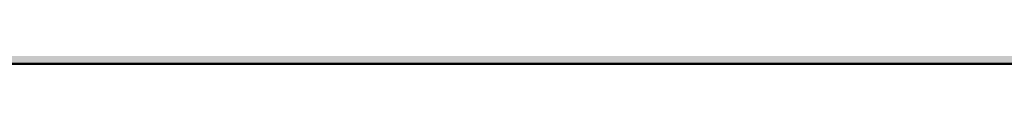
# Model space of a CAD drawing. Units: millimetres. Extents: x 0 to 2267, y 0 to 1823.
# Tile 160 of 256: x 1833.606 to 1838.83, y 1127.417 to 1127.417. Entities that reach past the tile are written whole.
import ezdxf

# ---------------------------------------------------------------- set-up
doc = ezdxf.new("R2010")
doc.units = ezdxf.units.MM
doc.header["$MEASUREMENT"] = 0
for name, color, linetype, lineweight in [('M-DIMS', 2, 'Continuous', 25), ('M-HATC', 252, 'Continuous', 18), ('M-OUTL', 7, 'Continuous', 50)]:
    doc.layers.add(name, color=color, linetype=linetype, lineweight=lineweight)
doc.styles.get("Standard").update_dxf_attribs({"font": 'arial.ttf'})
doc.dimstyles.get("Standard").update_dxf_attribs({"dimtxt": 7, "dimasz": 4, "dimexe": 0.18, "dimexo": 0.0625, "dimgap": 0.09, "dimtad": 0, "dimdec": 0, "dimzin": 0, "dimdsep": 46, "dimtxsty": 'Standard', "dimcen": 0.09, "dimadec": 0, "dimazin": 0, "dimtfac": 1, "dimtdec": 0, "dimtofl": 0, "dimtmove": 0, "dimatfit": 3, "dimfxl": 1, "dimtolj": 1, "dimtzin": 0, "dimarcsym": 0})

# ---------------------------------------------------------------- blocks, each defined once
blk = doc.blocks.new('*D1')
at = {"layer": 'Defpoints', "color": 0, "transparency": 16777216}
for p in [(1593.4289, 1127.4171), (1843.4289, 1127.4171), (1843.4289, 955.6278)]:
    blk.add_point(p, dxfattribs=at)
at = {"layer": 'M-DIMS', "color": 0, "lineweight": -2, "transparency": 16777216}
for p, q in [((1593.4289, 1127.3546), (1593.4289, 955.4478)), ((1843.4289, 1127.3546), (1843.4289, 955.4478)), ((1597.4289, 955.6278), (1710.5582, 955.6278)), ((1839.4289, 955.6278), (1726.2996, 955.6278))]:
    blk.add_line(p, q, dxfattribs=at)
at = {"layer": 'M-DIMS', "color": 0, "transparency": 16777216}
for points in [[(1597.4289, 956.2944), (1597.4289, 954.9611), (1593.4289, 955.6278)], [(1839.4289, 956.2944), (1839.4289, 954.9611), (1843.4289, 955.6278)]]:
    blk.add_solid(points, dxfattribs=at)
at = {"layer": 'M-DIMS', "color": 0, "transparency": 16777216, "insert": (1718.4289, 955.6278), "char_height": 7, "attachment_point": 5}
blk.add_mtext('\\A1;250', dxfattribs=at)

msp = doc.modelspace()

# ---------------------------------------------------------------- hatches: boundary and pattern name
at = {"layer": 'M-HATC'}
h = msp.add_hatch(color=256, dxfattribs=at)
h.dxf.hatch_style = 1
h.paths.add_polyline_path([(2042.8886, 1580.1796), (2055.771, 1593.062), (1381.0868, 1593.062), (1393.9692, 1580.1796), (1374.086, 1560.2964), (2062.7718, 1560.2964)])
h.paths.add_polyline_path([(1843.4289, 1201.3297), (1843.4289, 1227.2475), (1593.4289, 1227.2475), (1593.4289, 1201.3297, -0.228274), (1574.5989, 1162.2346), (1530.9289, 1127.4171), (1905.9289, 1127.4171), (1862.2589, 1162.2346, -0.228274)])

# ---------------------------------------------------------------- linework, layer by layer
at = {"layer": 'M-OUTL'}
msp.add_line((1530.9289, 1127.4171), (1905.9289, 1127.4171), dxfattribs=at)

# ---------------------------------------------------------------- dimensions: what is measured, and where the dimension line sits
at = {"layer": 'M-DIMS'}
dim = msp.add_linear_dim(base=(1843.4289, 955.6278), p1=(1593.4289, 1127.4171), p2=(1843.4289, 1127.4171), dimstyle='Standard', override={"dimclrd": 0, "dimclre": 0, "dimclrt": 0}, dxfattribs=at)
dim.commit()
dim.dimension.update_dxf_attribs({"geometry": '*D1', "text_midpoint": (1718.4289, 955.6278)})

doc.saveas('drawing.dxf')
